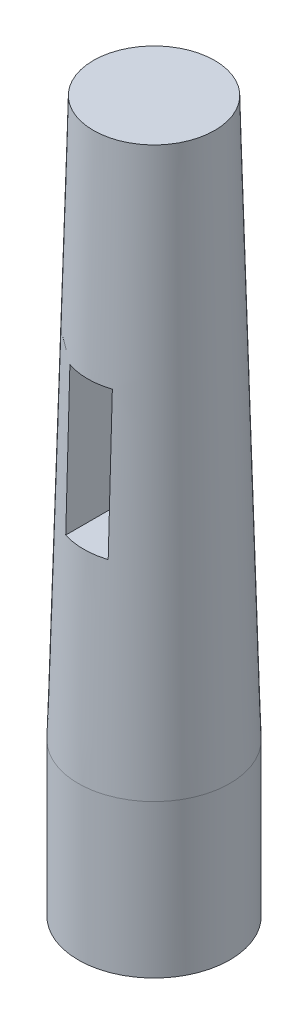
ISO-10303-21;
HEADER;
FILE_DESCRIPTION(('STEP AP214'),'2;1');
FILE_NAME('part.step','',(''),(''),'','','');
FILE_SCHEMA(('AUTOMOTIVE_DESIGN { 1 0 10303 214 1 1 1 1 }'));
ENDSEC;
DATA;
#1=APPLICATION_CONTEXT('core data for automotive mechanical design processes');
#2=APPLICATION_PROTOCOL_DEFINITION('international standard','automotive_design',2000,#1);
#3=PRODUCT_CONTEXT('',#1,'mechanical');
#4=PRODUCT('Part','Part','',(#3));
#5=PRODUCT_RELATED_PRODUCT_CATEGORY('part','',(#4));
#6=PRODUCT_DEFINITION_FORMATION('','',#4);
#7=PRODUCT_DEFINITION_CONTEXT('part definition',#1,'design');
#8=PRODUCT_DEFINITION('design','',#6,#7);
#9=PRODUCT_DEFINITION_SHAPE('','',#8);
#10=(LENGTH_UNIT() NAMED_UNIT(*) SI_UNIT(.MILLI.,.METRE.));
#11=(NAMED_UNIT(*) PLANE_ANGLE_UNIT() SI_UNIT($,.RADIAN.));
#12=(NAMED_UNIT(*) SI_UNIT($,.STERADIAN.) SOLID_ANGLE_UNIT());
#13=UNCERTAINTY_MEASURE_WITH_UNIT(LENGTH_MEASURE(1.E-05),#10,'distance_accuracy_value','');
#14=(GEOMETRIC_REPRESENTATION_CONTEXT(3) GLOBAL_UNCERTAINTY_ASSIGNED_CONTEXT((#13)) GLOBAL_UNIT_ASSIGNED_CONTEXT((#10,
#11,#12)) REPRESENTATION_CONTEXT('',''));
#15=CARTESIAN_POINT('',(0.,0.,0.));
#16=DIRECTION('',(0.,0.,1.));
#17=DIRECTION('',(1.,0.,0.));
#18=AXIS2_PLACEMENT_3D('',#15,#16,#17);
#19=CARTESIAN_POINT('',(0.,25.2,0.));
#20=DIRECTION('',(0.,-1.,0.));
#21=DIRECTION('',(0.,0.,-1.));
#22=AXIS2_PLACEMENT_3D('',#19,#20,#21);
#23=CYLINDRICAL_SURFACE('',#22,12.5);
#24=CARTESIAN_POINT('',(0.,25.2,0.));
#25=DIRECTION('',(0.,-1.,0.));
#26=DIRECTION('',(0.,0.,-1.));
#27=AXIS2_PLACEMENT_3D('',#24,#25,#26);
#28=CIRCLE('',#27,12.5);
#29=CARTESIAN_POINT('',(0.,25.2,-12.5));
#30=VERTEX_POINT('',#29);
#31=EDGE_CURVE('E113',#30,#30,#28,.F.);
#32=ORIENTED_EDGE('',*,*,#31,.F.);
#33=EDGE_LOOP('',(#32));
#34=FACE_BOUND('',#33,.T.);
#35=CARTESIAN_POINT('',(0.,0.,0.));
#36=DIRECTION('',(0.,1.,0.));
#37=DIRECTION('',(0.,0.,1.));
#38=AXIS2_PLACEMENT_3D('',#35,#36,#37);
#39=CIRCLE('',#38,12.5);
#40=CARTESIAN_POINT('',(0.,0.,12.5));
#41=VERTEX_POINT('',#40);
#42=EDGE_CURVE('E159',#41,#41,#39,.T.);
#43=ORIENTED_EDGE('',*,*,#42,.T.);
#44=EDGE_LOOP('',(#43));
#45=FACE_BOUND('',#44,.T.);
#46=ADVANCED_FACE('F43',(#34,#45),#23,.T.);
#47=CARTESIAN_POINT('',(0.,0.,0.));
#48=DIRECTION('',(0.,1.,0.));
#49=DIRECTION('',(0.,0.,1.));
#50=AXIS2_PLACEMENT_3D('',#47,#48,#49);
#51=PLANE('',#50);
#52=ORIENTED_EDGE('',*,*,#42,.F.);
#53=EDGE_LOOP('',(#52));
#54=FACE_BOUND('',#53,.T.);
#55=ADVANCED_FACE('F146',(#54),#51,.F.);
#56=CARTESIAN_POINT('',(0.,117.2,0.));
#57=DIRECTION('',(0.,1.,0.));
#58=DIRECTION('',(0.,0.,1.));
#59=AXIS2_PLACEMENT_3D('',#56,#57,#58);
#60=PLANE('',#59);
#61=CARTESIAN_POINT('',(0.,117.2,0.));
#62=DIRECTION('',(0.,1.,0.));
#63=DIRECTION('',(0.,0.,1.));
#64=AXIS2_PLACEMENT_3D('',#61,#62,#63);
#65=CIRCLE('',#64,10.);
#66=CARTESIAN_POINT('',(0.,117.2,10.));
#67=VERTEX_POINT('',#66);
#68=EDGE_CURVE('E161',#67,#67,#65,.T.);
#69=ORIENTED_EDGE('',*,*,#68,.T.);
#70=EDGE_LOOP('',(#69));
#71=FACE_BOUND('',#70,.T.);
#72=ADVANCED_FACE('F148',(#71),#60,.T.);
#73=CARTESIAN_POINT('',(0.,117.2,0.));
#74=DIRECTION('',(0.,-1.,0.));
#75=DIRECTION('',(0.,0.,-1.));
#76=AXIS2_PLACEMENT_3D('',#73,#74,#75);
#77=CONICAL_SURFACE('',#76,10.,0.0271672274043232);
#78=CARTESIAN_POINT('',(3.49999999999999,116.855646902327,-9.37748558964388));
#79=CARTESIAN_POINT('',(3.49999999999999,113.60879409088,-9.47166045559094));
#80=CARTESIAN_POINT('',(3.5,110.361936263016,-9.56566216155899));
#81=CARTESIAN_POINT('',(3.5,103.86821148013,-9.75334814651034));
#82=CARTESIAN_POINT('',(3.5,100.621344525108,-9.8470324254983));
#83=CARTESIAN_POINT('',(3.5,85.0695524547392,-10.2950683306127));
#84=CARTESIAN_POINT('',(3.5,72.7645717717569,-10.647492219225));
#85=CARTESIAN_POINT('',(3.5,54.30703512728,-11.1738356573649));
#86=CARTESIAN_POINT('',(3.5,48.1545117833693,-11.348901409721));
#87=CARTESIAN_POINT('',(3.5,35.849446064905,-11.6983607568969));
#88=CARTESIAN_POINT('',(3.50000000000001,29.6969036903515,-11.8727543517233));
#89=CARTESIAN_POINT('',(3.50000000000001,23.5443530976731,-12.0468578583962));
#90=B_SPLINE_CURVE_WITH_KNOTS('',3,(#78,#79,#80,#81,#82,#83,#84,#85,#86,#87,#88,#89),
.UNSPECIFIED.,.F.,.F.,(4,2,2,2,2,4),(0.,9.74465486652765,19.4893095897153,56.4193884034801,
74.8844289653302,93.3494693470719),.UNSPECIFIED.);
#91=CARTESIAN_POINT('',(3.5,82.2,-10.3767194011065));
#92=VERTEX_POINT('',#91);
#93=CARTESIAN_POINT('',(3.5,58.2,-11.0628053769007));
#94=VERTEX_POINT('',#93);
#95=EDGE_CURVE('E12',#92,#94,#90,.T.);
#96=ORIENTED_EDGE('',*,*,#95,.F.);
#97=CARTESIAN_POINT('',(0.,82.2,0.));
#98=DIRECTION('',(0.,1.,0.));
#99=DIRECTION('',(0.,0.,1.));
#100=AXIS2_PLACEMENT_3D('',#97,#98,#99);
#101=CIRCLE('',#100,10.9510869565217);
#102=CARTESIAN_POINT('',(-3.5,82.2,-10.3767194011065));
#103=VERTEX_POINT('',#102);
#104=EDGE_CURVE('E84',#103,#92,#101,.F.);
#105=ORIENTED_EDGE('',*,*,#104,.F.);
#106=CARTESIAN_POINT('',(-3.49999999999999,23.5443530976731,-12.0468578583962));
#107=CARTESIAN_POINT('',(-3.49999999999999,27.6138013560031,-11.9317025459048));
#108=CARTESIAN_POINT('',(-3.49999999999999,31.6832459788126,-11.8164189373675));
#109=CARTESIAN_POINT('',(-3.5,39.822127209442,-11.585571177381));
#110=CARTESIAN_POINT('',(-3.5,43.8915638172619,-11.4700070259359));
#111=CARTESIAN_POINT('',(-3.5,59.4435222360473,-11.0277790900016));
#112=CARTESIAN_POINT('',(-3.5,70.9260139584275,-10.7000553932185));
#113=CARTESIAN_POINT('',(-3.5,88.1496833324598,-10.206083798469));
#114=CARTESIAN_POINT('',(-3.5,93.8908952053111,-10.0410289219186));
#115=CARTESIAN_POINT('',(-3.5,105.373292159379,-9.70998879359023));
#116=CARTESIAN_POINT('',(-3.5,111.114477240595,-9.54400354180672));
#117=CARTESIAN_POINT('',(-3.50000000000001,116.855646902327,-9.37748558964391));
#118=B_SPLINE_CURVE_WITH_KNOTS('',3,(#106,#107,#108,#109,#110,#111,#112,#113,#114,#115,#116,
#117),.UNSPECIFIED.,.F.,.F.,(4,2,2,2,2,4),(0.,12.2132316992651,24.4264632260557,
58.8879655498637,76.1187174106417,93.3494693762124),.UNSPECIFIED.);
#119=CARTESIAN_POINT('',(-3.5,58.2,-11.0628053769007));
#120=VERTEX_POINT('',#119);
#121=EDGE_CURVE('E89',#120,#103,#118,.T.);
#122=ORIENTED_EDGE('',*,*,#121,.F.);
#123=CARTESIAN_POINT('',(0.,58.2,0.));
#124=DIRECTION('',(0.,-1.,0.));
#125=DIRECTION('',(0.,0.,-1.));
#126=AXIS2_PLACEMENT_3D('',#123,#124,#125);
#127=CIRCLE('',#126,11.6032608695652);
#128=EDGE_CURVE('E57',#94,#120,#127,.F.);
#129=ORIENTED_EDGE('',*,*,#128,.F.);
#130=EDGE_LOOP('',(#96,#105,#122,#129));
#131=FACE_BOUND('',#130,.T.);
#132=CARTESIAN_POINT('',(3.50000000000001,23.5443530976731,12.0468578583962));
#133=CARTESIAN_POINT('',(3.50000000000001,27.6138013560031,11.9317025459048));
#134=CARTESIAN_POINT('',(3.50000000000001,31.6832459788126,11.8164189373675));
#135=CARTESIAN_POINT('',(3.5,39.822127209442,11.585571177381));
#136=CARTESIAN_POINT('',(3.5,43.8915638172619,11.4700070259359));
#137=CARTESIAN_POINT('',(3.5,59.4435222360473,11.0277790900016));
#138=CARTESIAN_POINT('',(3.5,70.9260139584275,10.7000553932185));
#139=CARTESIAN_POINT('',(3.5,88.1496833324598,10.206083798469));
#140=CARTESIAN_POINT('',(3.5,93.8908952053111,10.0410289219186));
#141=CARTESIAN_POINT('',(3.5,105.373292159379,9.70998879359023));
#142=CARTESIAN_POINT('',(3.5,111.114477240595,9.54400354180672));
#143=CARTESIAN_POINT('',(3.49999999999999,116.855646902327,9.37748558964391));
#144=B_SPLINE_CURVE_WITH_KNOTS('',3,(#132,#133,#134,#135,#136,#137,#138,#139,#140,#141,#142,
#143),.UNSPECIFIED.,.F.,.F.,(4,2,2,2,2,4),(0.,12.2132316992651,24.4264632260557,
58.8879655498637,76.1187174106417,93.3494693762124),.UNSPECIFIED.);
#145=CARTESIAN_POINT('',(3.5,58.2,11.0628053769007));
#146=VERTEX_POINT('',#145);
#147=CARTESIAN_POINT('',(3.5,82.2,10.3767194011065));
#148=VERTEX_POINT('',#147);
#149=EDGE_CURVE('E93',#146,#148,#144,.T.);
#150=ORIENTED_EDGE('',*,*,#149,.F.);
#151=CARTESIAN_POINT('',(-3.5,58.2,11.0628053769007));
#152=VERTEX_POINT('',#151);
#153=EDGE_CURVE('E107',#152,#146,#127,.F.);
#154=ORIENTED_EDGE('',*,*,#153,.F.);
#155=CARTESIAN_POINT('',(-3.50000000000001,116.855646902327,9.37748558964388));
#156=CARTESIAN_POINT('',(-3.50000000000001,113.60879409088,9.47166045559093));
#157=CARTESIAN_POINT('',(-3.5,110.361936263016,9.56566216155898));
#158=CARTESIAN_POINT('',(-3.5,103.86821148013,9.75334814651033));
#159=CARTESIAN_POINT('',(-3.5,100.621344525108,9.8470324254983));
#160=CARTESIAN_POINT('',(-3.5,85.0695524547392,10.2950683306127));
#161=CARTESIAN_POINT('',(-3.5,72.7645717717569,10.647492219225));
#162=CARTESIAN_POINT('',(-3.5,54.30703512728,11.1738356573649));
#163=CARTESIAN_POINT('',(-3.5,48.1545117833693,11.348901409721));
#164=CARTESIAN_POINT('',(-3.5,35.849446064905,11.6983607568969));
#165=CARTESIAN_POINT('',(-3.49999999999999,29.6969036903515,11.8727543517233));
#166=CARTESIAN_POINT('',(-3.49999999999999,23.5443530976731,12.0468578583962));
#167=B_SPLINE_CURVE_WITH_KNOTS('',3,(#155,#156,#157,#158,#159,#160,#161,#162,#163,#164,#165,
#166),.UNSPECIFIED.,.F.,.F.,(4,2,2,2,2,4),(0.,9.74465486652765,19.4893095897153,
56.4193884034801,74.8844289653302,93.3494693470719),.UNSPECIFIED.);
#168=CARTESIAN_POINT('',(-3.5,82.2,10.3767194011065));
#169=VERTEX_POINT('',#168);
#170=EDGE_CURVE('E112',#169,#152,#167,.T.);
#171=ORIENTED_EDGE('',*,*,#170,.F.);
#172=EDGE_CURVE('E91',#148,#169,#101,.F.);
#173=ORIENTED_EDGE('',*,*,#172,.F.);
#174=EDGE_LOOP('',(#150,#154,#171,#173));
#175=FACE_BOUND('',#174,.T.);
#176=ORIENTED_EDGE('',*,*,#31,.T.);
#177=EDGE_LOOP('',(#176));
#178=FACE_BOUND('',#177,.T.);
#179=ORIENTED_EDGE('',*,*,#68,.F.);
#180=EDGE_LOOP('',(#179));
#181=FACE_BOUND('',#180,.T.);
#182=ADVANCED_FACE('F105',(#131,#175,#178,#181),#77,.T.);
#183=CARTESIAN_POINT('',(3.5,82.2,-17.6));
#184=DIRECTION('',(1.,0.,0.));
#185=DIRECTION('',(0.,1.,0.));
#186=AXIS2_PLACEMENT_3D('',#183,#184,#185);
#187=PLANE('',#186);
#188=ORIENTED_EDGE('',*,*,#95,.T.);
#189=DIRECTION('',(0.,0.,1.));
#190=VECTOR('',#189,1.);
#191=CARTESIAN_POINT('',(3.5,58.2,-17.6));
#192=LINE('',#191,#190);
#193=EDGE_CURVE('E164',#94,#146,#192,.T.);
#194=ORIENTED_EDGE('',*,*,#193,.T.);
#195=ORIENTED_EDGE('',*,*,#149,.T.);
#196=DIRECTION('',(0.,0.,1.));
#197=VECTOR('',#196,1.);
#198=CARTESIAN_POINT('',(3.5,82.2,-17.6));
#199=LINE('',#198,#197);
#200=EDGE_CURVE('E68',#92,#148,#199,.T.);
#201=ORIENTED_EDGE('',*,*,#200,.F.);
#202=EDGE_LOOP('',(#188,#194,#195,#201));
#203=FACE_BOUND('',#202,.T.);
#204=ADVANCED_FACE('F92',(#203),#187,.F.);
#205=CARTESIAN_POINT('',(-3.5,58.2,-17.6));
#206=DIRECTION('',(0.,-1.,0.));
#207=DIRECTION('',(0.,0.,-1.));
#208=AXIS2_PLACEMENT_3D('',#205,#206,#207);
#209=PLANE('',#208);
#210=ORIENTED_EDGE('',*,*,#153,.T.);
#211=ORIENTED_EDGE('',*,*,#193,.F.);
#212=ORIENTED_EDGE('',*,*,#128,.T.);
#213=DIRECTION('',(0.,0.,1.));
#214=VECTOR('',#213,1.);
#215=CARTESIAN_POINT('',(-3.5,58.2,-17.6));
#216=LINE('',#215,#214);
#217=EDGE_CURVE('E198',#120,#152,#216,.T.);
#218=ORIENTED_EDGE('',*,*,#217,.T.);
#219=EDGE_LOOP('',(#210,#211,#212,#218));
#220=FACE_BOUND('',#219,.T.);
#221=ADVANCED_FACE('F129',(#220),#209,.F.);
#222=CARTESIAN_POINT('',(-3.5,82.2,-17.6));
#223=DIRECTION('',(-1.,0.,0.));
#224=DIRECTION('',(0.,-1.,0.));
#225=AXIS2_PLACEMENT_3D('',#222,#223,#224);
#226=PLANE('',#225);
#227=ORIENTED_EDGE('',*,*,#170,.T.);
#228=ORIENTED_EDGE('',*,*,#217,.F.);
#229=ORIENTED_EDGE('',*,*,#121,.T.);
#230=DIRECTION('',(0.,0.,1.));
#231=VECTOR('',#230,1.);
#232=CARTESIAN_POINT('',(-3.5,82.2,-17.6));
#233=LINE('',#232,#231);
#234=EDGE_CURVE('E61',#103,#169,#233,.T.);
#235=ORIENTED_EDGE('',*,*,#234,.T.);
#236=EDGE_LOOP('',(#227,#228,#229,#235));
#237=FACE_BOUND('',#236,.T.);
#238=ADVANCED_FACE('F122',(#237),#226,.F.);
#239=CARTESIAN_POINT('',(-3.5,82.2,-17.6));
#240=DIRECTION('',(0.,1.,0.));
#241=DIRECTION('',(0.,0.,1.));
#242=AXIS2_PLACEMENT_3D('',#239,#240,#241);
#243=PLANE('',#242);
#244=ORIENTED_EDGE('',*,*,#104,.T.);
#245=ORIENTED_EDGE('',*,*,#200,.T.);
#246=ORIENTED_EDGE('',*,*,#172,.T.);
#247=ORIENTED_EDGE('',*,*,#234,.F.);
#248=EDGE_LOOP('',(#244,#245,#246,#247));
#249=FACE_BOUND('',#248,.T.);
#250=ADVANCED_FACE('F88',(#249),#243,.F.);
#251=CLOSED_SHELL('',(#46,#55,#72,#182,#204,#221,#238,#250));
#252=MANIFOLD_SOLID_BREP('B2',#251);
#253=ADVANCED_BREP_SHAPE_REPRESENTATION('',(#18,#252),#14);
#254=SHAPE_DEFINITION_REPRESENTATION(#9,#253);
ENDSEC;
END-ISO-10303-21;
